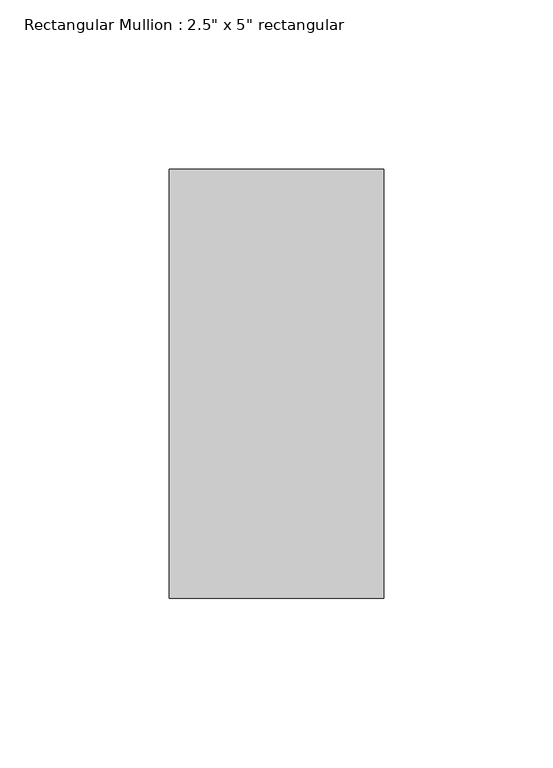
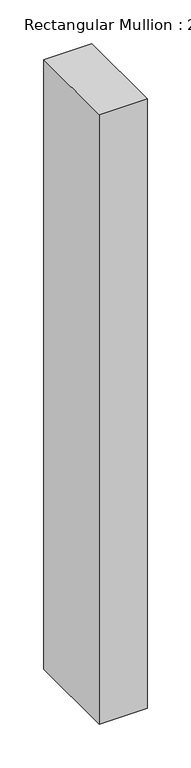
"""IFC4 building model written with IfcOpenShell, lengths in millimetres: member geometry."""

from ifc_helpers import new_model, si_unit, frame, origin, place, context, project, spatial, polyline, outline, extrude, source, transform, mapped, element, save


def member_39ae6cfa(model_context):
    return source(origin(), model_context, "Body", "SweptSolid", [
        extrude(outline(polyline([(0.0, 63.5), (0.0, -63.5), (-63.5, -63.5), (-63.5, 63.5), (0.0, 63.5)])), frame((0.0, 0.0, -851.313055), z_axis=(0.0, 0.0, 1.0), x_axis=(1.0, 0.0, 0.0)), (0.0, 0.0, 1.0), 851.313055),
    ])


if __name__ == "__main__":
    model = new_model("IFC4")
    model_context = context("Model", 3, world=origin())
    ifc_project = project(units=[si_unit("LENGTHUNIT", "METRE", prefix="MILLI")], contexts=[model_context])
    site = spatial("IfcSite", under=ifc_project)
    building = spatial("IfcBuilding", under=site)
    placement = place(None, origin())
    member_shape = member_39ae6cfa(model_context)
    element("IfcMember", 1, ObjectType="Rectangular Mullion : 2.5\" x 5\" rectangular", at=placement, inside=building, context=model_context, shape_type="MappedRepresentation", body=[
        mapped(member_shape, transform((0.0, 0.0, 0.0), x_axis=(1.0, 0.0, 0.0), y_axis=(0.0, 1.0, 0.0), z_axis=(0.0, 0.0, 1.0))),
    ])
    save(model, "model.ifc")

# Revit data of these elements
# Type "Rectangular Mullion : 2.5\" x 5\" rectangular"
#   built-in parameter 1007304 = 0.416667 (stored number, unit not read)
#   built-in parameter 1007301 = 0.104167 (stored number, unit not read)
#   built-in parameter 1007300 = 0.104167 (stored number, unit not read)
# Element 1 (IfcMember, "Rectangular Mullion : 2.5\" x 5\" rectangular")
#   Materials on its faces: "Aluminum"
# Materials
#   "Aluminum": class "Metal", colour RGB 247 247 247, transparency 0, Description = "Aluminum 6061", Cost = 0
